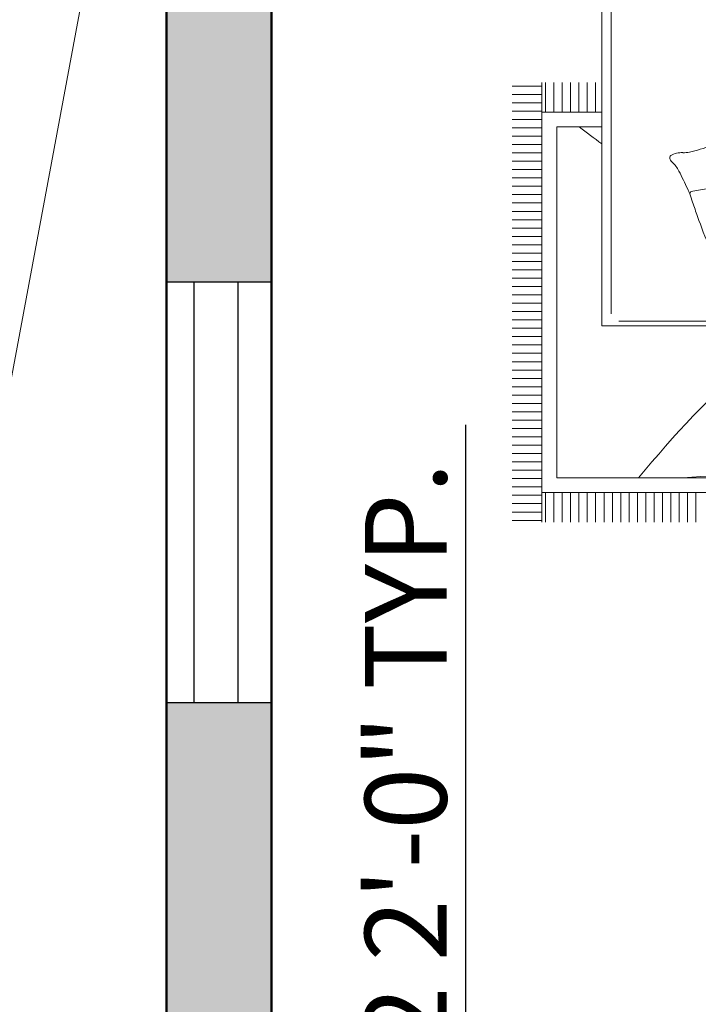
# Model space of a CAD drawing. Units: inches. Extents: x -7 to 1228, y -146 to 1091.
# Tile 27 of 88: x 621 to 680, y 362 to 446. Entities that reach past the tile are written whole.
import ezdxf

# ---------------------------------------------------------------- set-up
doc = ezdxf.new("R2010")
doc.units = ezdxf.units.IN
for name, color, linetype, lineweight in [('A-ANNO-DIMS', 2, 'Continuous', 18), ('A-FLOR-VOID', 7, 'Continuous', 18), ('A-FURN', 8, 'Continuous', 18), ('A-GLAZ', 175, 'Continuous', 25), ('A-WALL', 7, 'Continuous', 50), ('A-WALL-PATT', 251, 'Continuous', 13)]:
    doc.layers.add(name, color=color, linetype=linetype, lineweight=lineweight)
doc.styles.add('DIM_FONT', font='SIMPLEX.shx', dxfattribs={"width": 0.8})
doc.styles.get("Standard").update_dxf_attribs({"font": 'arial.ttf'})
doc.dimstyles.new('ISO-25', dxfattribs={"dimtxt": 7, "dimasz": 4, "dimexe": 1.25, "dimexo": 0.625, "dimtad": 1, "dimdec": 1, "dimlunit": 3, "dimtxsty": 'Standard', "dimcen": 2.5, "dimadec": 0, "dimazin": 0, "dimtfac": 1, "dimtdec": 1, "dimtmove": 1, "dimatfit": 3, "dimfxl": 1, "dimarcsym": 0})

# ---------------------------------------------------------------- blocks, each defined once
blk = doc.blocks.new('A$C4F634EDD')
for p, q in [((0.5, 0.5295), (0.5, 2.6295)), ((0.5258, 2.121), (0.5258, 0.5617)), ((0.2586, 1.1753), (0.3386, 1.1753)), ((0.3386, 0), (0.3386, 1.1852)), ((0.3486, 1.1052), (0.3486, 1.1852)), ((0.3711, 1.1052), (0.3711, 1.1852)), ((0.3936, 1.1052), (0.3936, 1.1852)), ((0.4161, 1.1052), (0.4161, 1.1852)), ((0.4386, 1.1052), (0.4386, 1.1852)), ((0.4611, 1.1052), (0.4611, 1.1852)), ((0.4836, 1.1052), (0.4836, 1.1852)), ((0.2586, 1.1528), (0.3386, 1.1528)), ((0.2586, 1.1303), (0.3386, 1.1303)), ((0.2586, 1.1078), (0.3386, 1.1078)), ((0.3386, 1.1052), (0.5, 1.1052)), ((0.2586, 1.0853), (0.3386, 1.0853)), ((0.2586, 1.0628), (0.3386, 1.0628)), ((0.3786, 1.0652), (0.5, 1.0652)), ((0.3786, 0.12), (0.3786, 1.0652)), ((0.2586, 1.0403), (0.3386, 1.0403)), ((0.2586, 1.0178), (0.3386, 1.0178)), ((0.2586, 0.9953), (0.3386, 0.9953)), ((0.2586, 0.9728), (0.3386, 0.9728)), ((0.2586, 0.9503), (0.3386, 0.9503)), ((0.2586, 0.9278), (0.3386, 0.9278)), ((0.2586, 0.9053), (0.3386, 0.9053)), ((0.8384, 0.9085), (0.7403, 0.8913)), ((0.2586, 0.8828), (0.3386, 0.8828)), ((0.7403, 0.8913), (0.737, 0.8849)), ((0.2586, 0.8603), (0.3386, 0.8603)), ((0.2586, 0.8378), (0.3386, 0.8378)), ((0.2586, 0.8153), (0.3386, 0.8153)), ((0.2586, 0.7928), (0.3386, 0.7928)), ((0.2586, 0.7703), (0.3386, 0.7703)), ((0.2586, 0.7478), (0.3386, 0.7478)), ((0.2586, 0.7253), (0.3386, 0.7253)), ((0.2586, 0.7028), (0.3386, 0.7028)), ((0.2586, 0.6803), (0.3386, 0.6803)), ((0.2586, 0.6578), (0.3386, 0.6578)), ((0.2586, 0.6353), (0.3386, 0.6353)), ((0.2586, 0.6128), (0.3386, 0.6128)), ((0.2586, 0.5903), (0.3386, 0.5903)), ((0.2586, 0.5678), (0.3386, 0.5678)), ((0.2586, 0.5453), (0.3386, 0.5453)), ((0.5458, 0.5417), (2.2516, 0.5417)), ((0.2586, 0.5228), (0.3386, 0.5228)), ((2.3, 0.5295), (0.5, 0.5295)), ((0.2586, 0.5003), (0.3386, 0.5003)), ((0.2586, 0.4778), (0.3386, 0.4778)), ((0.2586, 0.4553), (0.3386, 0.4553)), ((0.2586, 0.4328), (0.3386, 0.4328)), ((0.2586, 0.4103), (0.3386, 0.4103)), ((0.2586, 0.3878), (0.3386, 0.3878)), ((0.2586, 0.3653), (0.3386, 0.3653)), ((0.2586, 0.3428), (0.3386, 0.3428)), ((0.2586, 0.3203), (0.3386, 0.3203)), ((0.2586, 0.2978), (0.3386, 0.2978)), ((0.2586, 0.2753), (0.3386, 0.2753)), ((0.2586, 0.2528), (0.3386, 0.2528)), ((0.2586, 0.2303), (0.3386, 0.2303)), ((0.2586, 0.2078), (0.3386, 0.2078)), ((0.2586, 0.1853), (0.3386, 0.1853)), ((0.2586, 0.1628), (0.3386, 0.1628)), ((0.2586, 0.1403), (0.3386, 0.1403)), ((0.2586, 0.1178), (0.3386, 0.1178)), ((2.4188, 0.12), (0.3786, 0.12)), ((0.2586, 0.0953), (0.3386, 0.0953)), ((2.4588, 0.08), (0.3386, 0.08)), ((0.3486, 0), (0.3486, 0.08)), ((0.3711, 0), (0.3711, 0.08)), ((0.3936, 0), (0.3936, 0.08)), ((0.4161, 0), (0.4161, 0.08)), ((0.4386, 0), (0.4386, 0.08)), ((0.4611, 0), (0.4611, 0.08)), ((0.4836, 0), (0.4836, 0.08)), ((0.5061, 0), (0.5061, 0.08)), ((0.5286, 0), (0.5286, 0.08)), ((0.5511, 0), (0.5511, 0.08)), ((0.5736, 0), (0.5736, 0.08)), ((0.5961, 0), (0.5961, 0.08)), ((0.6186, 0), (0.6186, 0.08)), ((0.6411, 0), (0.6411, 0.08)), ((0.6636, 0), (0.6636, 0.08)), ((0.6861, 0), (0.6861, 0.08)), ((0.7086, 0), (0.7086, 0.08)), ((0.7311, 0), (0.7311, 0.08)), ((0.7536, 0), (0.7536, 0.08)), ((0.2586, 0.0728), (0.3386, 0.0728)), ((0.2586, 0.0503), (0.3386, 0.0503)), ((0.2586, 0.0278), (0.3386, 0.0278)), ((0.2586, 0.0053), (0.3386, 0.0053))]:
    blk.add_line(p, q)
for centre, radius, start, end in [((0.6422, 1.4168), 0.43, 282.6252, 290.7486), ((0.6894, 0.9832), 0.0058, 121.6917, 179.0386), ((0.7004, 0.983), 0.0168, 179.0386, 229.4914), ((0.7131, 0.9448), 0.0509, 103.0402, 121.6917), ((0.7152, 0.9361), 0.0599, 86.6119, 103.0402), ((0.7224, 1.0587), 0.063, 266.6119, 282.6252), ((0.6405, 0.9128), 0.0755, 26.3332, 49.4914), ((-1.6775, -0.2344), 2.6619, 25.1732, 26.3332), ((0.5689, 0.8213), 0.1798, 20.7081, 25.1732), ((0.2268, 0.692), 0.5454, 18.2369, 20.7081), ((2.3102, 1.3785), 1.6481, 198.2369, 199.6584), ((2.6444, 1.4979), 2.003, 199.6584, 202.2355)]:
    blk.add_arc(centre, radius, start, end)
blk.add_open_spline([(0.4393, 1.0652), (0.4595, 1.05), (0.4798, 1.0348), (0.5, 1.0195)], degree=3)
for points, knots in [([(0.5992, 0.12), (0.6957, 0.2341), (0.8523, 0.4189), (1.0536, 0.5069), (1.136, 0.5295)], [0, 0, 0, 0, 432.822832, 701.445452, 701.445452, 701.445452, 701.445452]), ([(0.7187, 0.12), (0.9791, 0.1362), (1.326, 0.1577), (1.3868, 0.4574), (1.408, 0.5295)], [0, 0, 0, 0, 653.160442, 870.050857, 870.050857, 870.050857, 870.050857])]:
    blk.add_open_spline(points, degree=3, knots=knots)
at = {"style": 'DIM_FONT', "width": 0.8, "flags": 9}
for tag, p in [('YSIZE', (0.5, 2.6295)), ('XSIZE', (0.5, 2.6295)), ('XSIZE', (2.2985, 2.6295)), ('YSIZE', (2.2985, 2.6295))]:
    blk.add_attdef(tag, p, '', height=0.0005, dxfattribs=at)
blk = doc.blocks.new('WIN-36')
for p, q in [((0, 36), (0, 0)), ((9, 36), (0, 36)), ((2.343, 36), (2.343, 0)), ((6.137, 0), (6.137, 36)), ((9, 0), (9, 36)), ((0, 0), (9, 0)), ((2.343, 0), (6.137, 0))]:
    blk.add_line(p, q)
blk = doc.blocks.new('*D50')
at = {"layer": 'A-ANNO-DIMS', "color": 0, "lineweight": -2, "transparency": 16777216}
for p, q in [((659.653, 304.545), (659.653, 411.76)), ((643.625, 312.629), (647.85, 312.629)), ((646.6, 292.629), (646.6, 308.629)), ((646.6, 300.629), (659.653, 304.545)), ((643.625, 288.629), (647.85, 288.629))]:
    blk.add_line(p, q, dxfattribs=at)
at = {"layer": 'A-ANNO-DIMS', "color": 0, "transparency": 16777216}
for points in [[(645.933, 308.629), (647.267, 308.629), (646.6, 312.629)], [(645.933, 292.629), (647.267, 292.629), (646.6, 288.629)]]:
    blk.add_solid(points, dxfattribs=at)
at = {"layer": 'Defpoints', "color": 0, "transparency": 16777216}
for p in [(643, 312.629), (646.6, 312.629), (643, 288.629)]:
    blk.add_point(p, dxfattribs=at)
at = {"layer": 'A-ANNO-DIMS', "color": 0, "transparency": 16777216, "insert": (655.406, 358.152), "char_height": 7, "attachment_point": 5, "rotation": 90}
blk.add_mtext('WINDOW W2 2\'-0" TYP.', dxfattribs=at)

msp = doc.modelspace()

# ---------------------------------------------------------------- hatches: boundary and pattern name
at = {"layer": 'A-WALL-PATT'}
h = msp.add_hatch(color=256, dxfattribs=at)
h.dxf.hatch_style = 1
h.paths.add_polyline_path([(69, 568), (60, 568), (60, 493), (63.289, 493), (69, 493)])
h.paths.add_polyline_path([(69, 662.405), (60, 662.405), (60, 586), (69, 586)], flags=17)
h.paths.add_polyline_path([(69, 723), (184, 723), (184, 734), (179, 734), (179, 728), (69, 728), (69, 741.623), (60, 741.623), (60, 698.405), (69, 698.405)], flags=17)
h.paths.add_polyline_path([(69, 782), (231, 782), (231, 728), (231, 723), (231, 586), (236, 586), (236, 787), (69, 787), (69, 800.126), (60, 800.126), (60, 765.623), (69, 765.623)])
h.paths.add_polyline_path([(184, 842), (189, 842), (189, 848), (173, 848), (173, 842), (179, 842), (179, 787), (184, 787)])
h.paths.add_polyline_path([(118.22, 69), (69, 69), (69, 60), (118.22, 60)])
h.paths.add_polyline_path([(227, 69), (154.22, 69), (154.22, 60), (227, 60)])
h.paths.add_polyline_path([(236, 60), (232.711, 60), (227, 60), (227, 36), (236, 36)])
h.paths.add_polyline_path([(389, 60), (380, 60), (380, 36), (389, 36)])
h.paths.add_polyline_path([(384, 181), (380, 181), (380, 115), (380, 78), (384, 78)])
h.paths.add_polyline_path([(380, 115), (334.547, 115), (334.547, 109), (380, 109)])
h.paths.add_polyline_path([(274.547, 115), (236, 115), (236, 201), (232.711, 201), (231, 201), (231, 78), (236, 78), (236, 109), (274.547, 109)])
h.paths.add_polyline_path([(69, 123), (60, 123), (60, 78), (69, 78)])
h.paths.add_polyline_path([(69, 201), (60, 201), (60, 159), (69, 159)])
h.paths.add_polyline_path([(143, 219), (69, 219), (69, 213), (143, 213)], flags=17)
h.paths.add_polyline_path([(189, 219), (184, 219), (184, 274), (231, 274), (231, 219), (236, 219), (236, 279), (184, 279), (184, 297), (179, 297), (179, 279), (69, 279), (69, 290.912), (60, 290.912), (60, 262.179), (69, 262.179), (69, 274), (179, 274), (179, 219), (173, 219), (173, 213), (189, 213)])
h.paths.add_polyline_path([(69, 238.179), (60, 238.179), (60, 219), (69, 219)], flags=17)
h.paths.add_polyline_path([(69, 333), (60, 333), (60, 314.912), (69, 314.912), (69, 316.965)])
h.paths.add_polyline_path([(190, 338), (184, 338), (69, 338), (69, 333), (179, 333), (179, 327), (184, 327), (184, 333.021), (190, 333.046)])
h.paths.add_polyline_path([(69, 386.806), (60, 386.806), (60, 351), (69, 351)])
h.paths.add_polyline_path([(69, 475), (60, 475), (60, 422.806), (69, 422.806)])
h.paths.add_polyline_path([(236, 475), (231, 475), (231, 351.238), (236, 351.238)])
h.paths.add_polyline_path([(384, 475), (380, 475), (380, 362), (384, 362)])
h.paths.add_polyline_path([(547, 307), (439, 307), (439, 356), (445, 356), (445, 362), (433, 362), (433, 307), (380, 307), (380, 244), (380, 241), (384, 241), (384, 301), (433, 301), (433, 277), (439, 277), (439, 301), (547, 301)])
h.paths.add_polyline_path([(547, 241), (439, 241), (439, 247), (433, 247), (433, 235), (547, 235)])
h.paths.add_polyline_path([(450, 69), (440.286, 69), (424.889, 69), (389, 69), (389, 60), (450, 60)])
h.paths.add_polyline_path([(547, 69), (486, 69), (486, 60), (547, 60)])
h.paths.add_polyline_path([(556, 148.268), (547, 148.268), (547, 78), (556, 78)])
h.paths.add_polyline_path([(556, 223), (547, 223), (547, 195), (547, 184.268), (556, 184.268)])
h.paths.add_polyline_path([(556, 311.192), (547, 311.192), (547, 273.075), (556, 273.075)])
h.paths.add_polyline_path([(556, 344), (552.711, 344), (547, 344), (547, 335.192), (556, 335.192)])
h.paths.add_polyline_path([(556, 249.075), (547, 249.075), (547, 241), (556, 241)])
h.paths.add_polyline_path([(547, 362), (475, 362), (475, 356), (547, 356)], flags=0)
h.paths.add_polyline_path([(556, 399.621), (547, 399.621), (547, 362), (556, 362)])
h.paths.add_polyline_path([(556, 475), (547, 475), (547, 435.621), (556, 435.621)])
h.paths.add_polyline_path([(547, 493), (389, 493), (389, 487), (547, 487)])
h.paths.add_polyline_path([(380, 493), (278, 493), (278, 487), (380, 487)])
h.paths.add_polyline_path([(227, 493), (69, 493), (69, 487), (227, 487)])
h.paths.add_polyline_path([(643, 122.445), (634, 122.445), (634, 78), (643, 78)])
h.paths.add_polyline_path([(702.5, 69), (692.786, 69), (677.389, 69), (643, 69), (643, 60), (702.5, 60)])
h.paths.add_polyline_path([(798, 69), (738.5, 69), (738.5, 60), (798, 60)])
h.paths.add_polyline_path([(807, 60), (803.711, 60), (798, 60), (798, 36), (807, 36)])
h.paths.add_polyline_path([(807, 109), (846.751, 109), (846.751, 115), (807, 115), (807, 159), (802, 159), (802, 78), (807, 78)])
h.paths.add_polyline_path([(807, 201), (802, 201), (802, 195), (807, 195)])
h.paths.add_polyline_path([(643, 201), (634, 201), (634, 158.445), (643, 158.445)])
h.paths.add_polyline_path([(756, 225), (751, 225), (751, 219), (643, 219), (643, 213), (756, 213)])
h.paths.add_polyline_path([(643, 240.848), (634, 240.848), (634, 219), (643, 219)])
h.paths.add_polyline_path([(643, 274), (643, 288.629), (634, 288.629), (634, 264.848), (643, 264.848)])
h.paths.add_polyline_path([(802, 279), (756, 279), (756, 297), (751, 297), (751, 279), (643, 279), (643, 274), (751, 274), (751, 255), (756, 255), (756, 274), (802, 274)])
h.paths.add_polyline_path([(807, 333), (803.711, 333), (802, 333), (802, 279), (802, 274), (802, 219), (807, 219)])
h.paths.add_polyline_path([(956, 182), (951, 182), (951, 115), (906.751, 115), (906.751, 109), (951, 109), (951, 78), (956, 78)])
h.paths.add_polyline_path([(960, 60), (951, 60), (951, 36), (960, 36)])
h.paths.add_polyline_path([(1021, 69), (1005.781, 69), (960, 69), (960, 60), (1021, 60)])
h.paths.add_polyline_path([(956, 224), (951, 224), (951, 218), (956, 218)])
h.paths.add_polyline_path([(956, 302), (1004, 302), (1004, 278), (1010, 278), (1010, 302), (1118, 302), (1118, 290.809), (1127, 290.809), (1127, 326.968), (1118, 326.968), (1118, 320.966), (1118, 307), (1010, 307), (1010, 356), (1016, 356), (1016, 362), (1004, 362), (1004, 307), (951, 307), (951, 244), (951, 242), (954.289, 242), (956, 242)])
h.paths.add_polyline_path([(643, 333), (634, 333), (634, 312.629), (643, 312.629), (643, 316.965)])
h.paths.add_polyline_path([(756, 338), (643, 338), (643, 333), (751, 333), (751, 327), (756, 327)])
h.paths.add_polyline_path([(643, 388), (634, 388), (634, 351), (643, 351)])
h.paths.add_polyline_path([(807, 357), (802, 357), (802, 351), (807, 351)])
h.paths.add_polyline_path([(807, 475), (802, 475), (802, 393), (807, 393)])
h.paths.add_polyline_path([(643, 475), (634, 475), (634, 424), (643, 424)])
h.paths.add_polyline_path([(798, 493), (643, 493), (643, 487), (798, 487)])
h.paths.add_polyline_path([(634, 493), (556, 493), (556, 487), (634, 487)])
h.paths.add_polyline_path([(813, 493), (807, 493), (807, 487), (813, 487)])
h.paths.add_polyline_path([(951, 493), (849, 493), (849, 487), (951, 487)])
h.paths.add_polyline_path([(956, 484), (951, 484), (951, 374), (956, 374)])
h.paths.add_polyline_path([(1109, 493), (969, 493), (969, 487), (1109, 487)])
h.paths.add_polyline_path([(1127, 484), (1118, 484), (1118, 450.641), (1127, 450.641)])
h.paths.add_polyline_path([(1127, 414.641), (1118, 414.641), (1118, 365), (1127, 365)])
h.paths.add_polyline_path([(1109, 362), (1046, 362), (1046, 356), (1109, 356)], flags=17)
h.paths.add_polyline_path([(1127, 356), (1123.454, 356), (1118, 356), (1118, 350.968), (1127, 350.968)], flags=0)
h.paths.add_polyline_path([(1127, 266.809), (1118, 266.809), (1118, 262.361), (1118, 242), (1127, 242)], flags=17)
h.paths.add_polyline_path([(1118, 242), (1010, 242), (1010, 248), (1004, 248), (1004, 237), (1118, 237)])
h.paths.add_polyline_path([(1127, 224), (1118, 224), (1118, 170), (1127, 170)])
h.paths.add_polyline_path([(1127, 134), (1118, 134), (1118, 78), (1127, 78)])
h.paths.add_polyline_path([(1118, 69), (1057, 69), (1057, 60), (1118, 60)])
h.paths.add_polyline_path([(227, 571.546), (227, 574), (69, 574), (69, 568), (227, 568)])
h.paths.add_polyline_path([(380, 571.546), (380, 574), (278, 574), (278, 568), (380, 568)])
h.paths.add_polyline_path([(242, 574), (236, 574), (236, 568), (242, 568)])
h.paths.add_polyline_path([(547, 571.546), (547, 574), (389, 574), (389, 568), (547, 568)])
h.paths.add_polyline_path([(384, 733), (380, 733), (380, 586), (384, 586)])
h.paths.add_polyline_path([(556, 646), (634, 646), (634, 655), (547, 655), (547, 586), (556, 586)])
h.paths.add_polyline_path([(634, 574), (556, 574), (556, 568), (634, 568)])
h.paths.add_polyline_path([(643, 655), (634, 655), (634, 586), (643, 586)])
h.paths.add_polyline_path([(798, 574), (643, 574), (643, 568), (798, 568)])
h.paths.add_polyline_path([(643, 663.854), (634, 663.854), (634, 655), (643, 655)])
h.paths.add_polyline_path([(556, 676.967), (547, 676.967), (547, 655), (556, 655)])
h.paths.add_polyline_path([(556, 733), (547, 733), (547, 712.967), (556, 712.967)])
h.paths.add_polyline_path([(643, 710), (634, 710), (634, 699.854), (643, 699.854)])
h.paths.add_polyline_path([(807, 668), (802, 668), (802, 586), (807, 586)])
h.paths.add_polyline_path([(951, 574), (849, 574), (849, 568), (951, 568)])
h.paths.add_polyline_path([(956, 691), (951, 691), (951, 577), (956, 577)])
h.paths.add_polyline_path([(1109, 574), (969, 574), (969, 568), (1109, 568)])
h.paths.add_polyline_path([(1127, 643.403), (1118, 643.403), (1118, 577), (1127, 577)])
h.paths.add_polyline_path([(1127, 568), (1123.454, 568), (1118, 568), (1118, 493), (1127, 493)])
h.paths.add_polyline_path([(1127, 733), (1118, 733), (1118, 679.403), (1127, 679.403)])
h.paths.add_polyline_path([(1127, 777.348), (1118, 777.348), (1118, 770.035), (1118, 751), (1127, 751)], flags=17)
h.paths.add_polyline_path([(1118, 751), (1010, 751), (1010, 757), (1004, 757), (1004, 745), (1118, 745)])
h.paths.add_polyline_path([(956, 811), (1004, 811), (1004, 787), (1010, 787), (1010, 811), (1017.874, 811), (1017.874, 811.627, -0.414214), (1018.247, 812), (1031.978, 812, -0.414214), (1032.351, 811.627), (1032.351, 811), (1118, 811), (1118, 801.348), (1127, 801.348), (1127, 834.685), (1118, 834.685), (1118, 830.238), (1118, 817), (1010, 817), (1010, 866), (1016, 866), (1016, 872), (1004, 872), (1004, 817), (956, 817), (956, 866), (951, 866), (951, 751), (954.289, 751), (956, 751)])
h.paths.add_polyline_path([(1118, 872), (1046, 872), (1046, 866), (1118, 866)], flags=17)
h.paths.add_polyline_path([(1127, 924.711), (1118, 924.711), (1118, 884), (1127, 884)])
h.paths.add_polyline_path([(1127, 866), (1123.711, 866), (1118, 866), (1118, 858.685), (1127, 858.685)], flags=17)
h.paths.add_polyline_path([(956, 983), (951, 983), (951, 952), (807, 952), (807, 983), (802, 983), (802, 902), (807, 902), (807, 946), (951, 946), (951, 884), (956, 884)])
h.paths.add_polyline_path([(807, 842), (802, 842), (802, 787), (756, 787), (756, 806), (751, 806), (751, 787), (643, 787), (643, 782), (751, 782), (751, 764), (756, 764), (756, 782), (802, 782), (802, 728), (807, 728)])
h.paths.add_polyline_path([(756, 848), (643, 848), (643, 842), (751, 842), (751, 836), (756, 836)])
h.paths.add_polyline_path([(756, 734), (751, 734), (751, 728), (643, 728), (643, 723), (756, 723)])
h.paths.add_polyline_path([(643, 749.791), (634, 749.791), (634, 728), (637.289, 728), (643, 728)])
h.paths.add_polyline_path([(643, 805.405), (634, 805.405), (634, 773.791), (643, 773.791)])
h.paths.add_polyline_path([(643, 896.663), (634, 896.663), (634, 860), (637.289, 860), (643, 860)])
h.paths.add_polyline_path([(643, 842), (634, 842), (634, 829.405), (643, 829.405)])
h.paths.add_polyline_path([(643, 983), (634, 983), (634, 932.663), (643, 932.663)])
h.paths.add_polyline_path([(1127, 983), (1118, 983), (1118, 960.711), (1127, 960.711)])
h.paths.add_polyline_path([(1118, 1001), (1077.525, 1001), (1077.525, 992), (1118, 992)])
h.paths.add_polyline_path([(1041.525, 1001), (960, 1001), (960, 992), (1041.525, 992)])
h.paths.add_polyline_path([(960, 1025), (951, 1025), (951, 1001), (954.289, 1001), (960, 1001)])
h.paths.add_polyline_path([(807, 1025), (798, 1025), (798, 1001), (807, 1001)])
h.paths.add_polyline_path([(798, 1001), (738.5, 1001), (738.5, 992), (798, 992)])
h.paths.add_polyline_path([(702.5, 1001), (643, 1001), (643, 992), (702.5, 992)])
h.paths.add_polyline_path([(547, 1001), (499.113, 1001), (499.113, 992), (547, 992)])
h.paths.add_polyline_path([(463.113, 1001), (389, 1001), (389, 992), (463.113, 992)])
h.paths.add_polyline_path([(389, 1025), (380, 1025), (380, 1022), (380, 1001), (383.289, 1001), (389, 1001)])
h.paths.add_polyline_path([(236, 1025), (227, 1025), (227, 1001), (236, 1001)])
h.paths.add_polyline_path([(236, 983), (231, 983), (231, 860), (236, 860)])
h.paths.add_polyline_path([(274.547, 952), (236, 952), (236, 946), (274.547, 946)])
h.paths.add_polyline_path([(380, 952), (334.547, 952), (334.547, 946), (380, 946)])
h.paths.add_polyline_path([(384, 983), (380, 983), (380, 884), (383.289, 884), (384, 884)])
h.paths.add_polyline_path([(227, 1001), (155.012, 1001), (155.012, 992), (162.875, 992), (227, 992)])
h.paths.add_polyline_path([(119.012, 1001), (69, 1001), (69, 992), (119.012, 992)])
h.paths.add_polyline_path([(69, 983), (60, 983), (60, 922.987), (69, 922.987)])
h.paths.add_polyline_path([(69, 886.987), (60, 886.987), (60, 860), (63.289, 860), (69, 860)])
h.paths.add_polyline_path([(143, 848), (69, 848), (69, 842), (143, 842)])

# ---------------------------------------------------------------- linework, layer by layer
at = {"layer": 'A-FLOR-VOID'}
msp.add_line((634, 487), (556, 69), dxfattribs=at)
at = {"layer": 'A-WALL'}
for p, q in [((634, 415), (634, 493)), ((634, 493), (634, 60)), ((643, 338), (643, 493)), ((643, 493), (643, 60)), ((634, 60), (634, 406))]:
    msp.add_line(p, q, dxfattribs=at)

# ---------------------------------------------------------------- block references
at = {"layer": 'A-FURN', "xscale": 31.78426361944092, "yscale": 31.78426361944092, "zscale": 31.78426361944092}
msp.add_blockref('A$C4F634EDD', (655.397, 403.423), dxfattribs=at)
at = {"layer": 'A-GLAZ'}
msp.add_blockref('WIN-36', (634, 388), dxfattribs=at)

# ---------------------------------------------------------------- dimensions: what is measured, and where the dimension line sits
at = {"layer": 'A-ANNO-DIMS'}
dim = msp.add_linear_dim(base=(646.6, 312.629), p1=(643, 288.629), p2=(643, 312.629), angle=90, text='WINDOW W2 <> TYP.', dimstyle='ISO-25', override={"dimdec": 1, "dimlfac": 1, "dimrnd": 0, "dimzin": 1, "dimdsep": 46, "dimlunit": 4, "dimfrac": 2}, dxfattribs=at)
dim.commit()
dim.dimension.update_dxf_attribs({"geometry": '*D50', "text_midpoint": (655.406, 305.17)})

doc.saveas('drawing.dxf')
